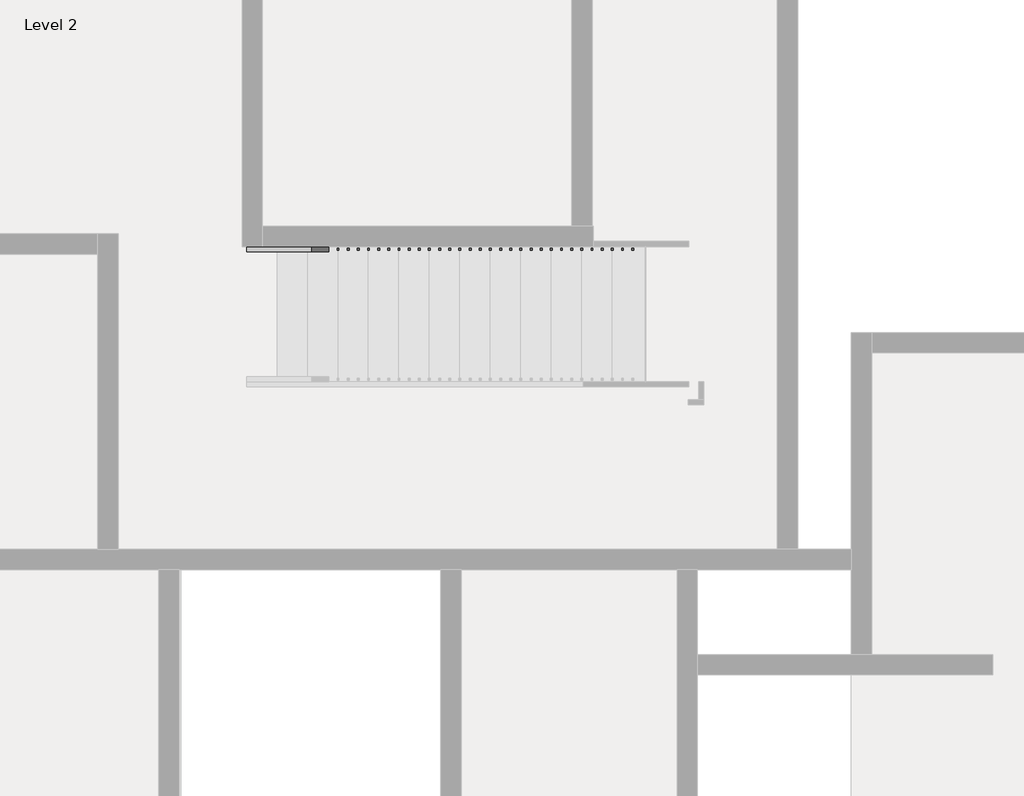
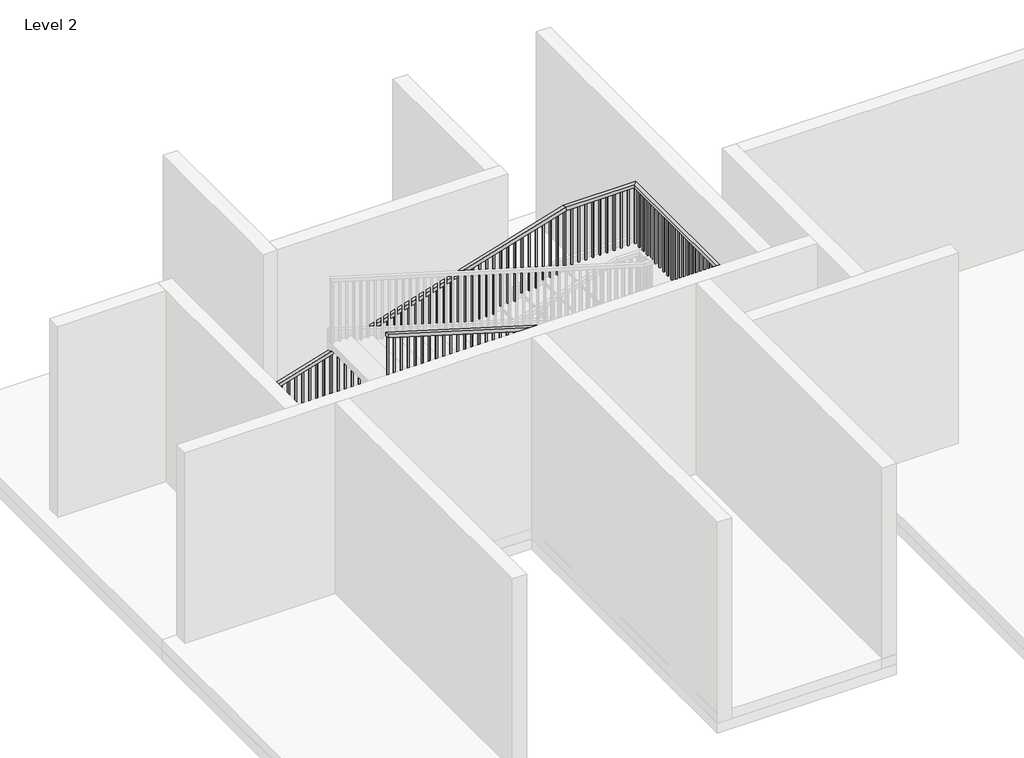
# One storey, part 10 of 14: 1 railing.
"""IFC4 building model written with IfcOpenShell, lengths in millimetres."""

from ifc_helpers import new_model, si_unit, frame, origin, place, context, project, spatial, polyline, outline, extrude, faceted_brep, element, save

model = new_model("IFC4")

# Units and contexts
model_context = context("Model", 3, world=origin())
ifc_project = project(units=[si_unit("LENGTHUNIT", "METRE", prefix="MILLI")], contexts=[model_context])

# Site, building, storey
site = spatial("IfcSite", under=ifc_project)
building = spatial("IfcBuilding", under=site)
storey = spatial("IfcBuildingStorey", under=building, Name="Level 2", Elevation=3048.0)

# Railing
placement = place(None, origin())
element("IfcRailing", 1, ObjectType="Handrail - Rectangular", at=placement, inside=storey, context=model_context, shape_type="SolidModel", body=[
    faceted_brep([(-5254.0891351, 12506.0715905, 4053.84), (-5254.0891351, 12506.0715905, 4000.8032429), (-5254.0891351, 12455.2715905, 4000.8032429), (-5254.0891351, 12455.2715905, 4053.84), (-986.8891351, 12506.0715905, 5334.0), (-979.4332782, 12506.0715905, 5283.2), (-979.4332782, 12455.2715905, 5283.2), (-986.8891351, 12455.2715905, 5334.0), (54.5108649, 12506.0715905, 5334.0), (54.5108649, 12506.0715905, 5283.2), (3.7108649, 12455.2715905, 5283.2), (3.7108649, 12455.2715905, 5334.0), (54.5108649, 9478.4949943, 5334.0), (54.5108649, 9478.4949943, 5283.2), (3.7108649, 9529.2949943, 5283.2), (3.7108649, 9529.2949943, 5334.0), (-682.0891351, 9478.4949943, 5334.0), (-689.544992, 9478.4949943, 5283.2), (-689.544992, 9529.2949943, 5283.2), (-682.0891351, 9529.2949943, 5334.0), (-5254.0891351, 9478.4949943, 6705.6), (-5254.0891351, 9529.2949943, 6705.6), (-5254.0891351, 9529.2949943, 6652.5632429), (-5254.0891351, 9478.4949943, 6652.5632429)], [[[0, 1, 2, 3]], [[1, 0, 4, 5]], [[2, 1, 5, 6]], [[3, 2, 6, 7]], [[0, 3, 7, 4]], [[5, 4, 8, 9]], [[6, 5, 9, 10]], [[7, 6, 10, 11]], [[4, 7, 11, 8]], [[9, 8, 12, 13]], [[10, 9, 13, 14]], [[11, 10, 14, 15]], [[8, 11, 15, 12]], [[13, 12, 16, 17]], [[14, 13, 17, 18]], [[15, 14, 18, 19]], [[12, 15, 19, 16]], [[20, 21, 22, 23]], [[17, 16, 20, 23]], [[18, 17, 23, 22]], [[19, 18, 22, 21]], [[16, 19, 21, 20]]]),
    extrude(outline(polyline([(6624.9407429, -5162.0141351), (5699.76, -5162.0141351), (5699.76, -5142.9641351), (6619.2257429, -5142.9641351), (6624.9407429, -5162.0141351)])), frame((0.0, 9494.3699943, 0.0), z_axis=(0.0, 1.0, 0.0), x_axis=(0.0, 0.0, 1.0)), (0.0, 0.0, 1.0), 19.05),
    extrude(outline(polyline([(6594.4607429, -5060.4141351), (5699.76, -5060.4141351), (5699.76, -5041.3641351), (6588.7457429, -5041.3641351), (6594.4607429, -5060.4141351)])), frame((0.0, 9494.3699943, 0.0), z_axis=(0.0, 1.0, 0.0), x_axis=(0.0, 0.0, 1.0)), (0.0, 0.0, 1.0), 19.05),
    extrude(outline(polyline([(6563.9807429, -4958.8141351), (5699.76, -4958.8141351), (5699.76, -4939.7641351), (6558.2657429, -4939.7641351), (6563.9807429, -4958.8141351)])), frame((0.0, 9494.3699943, 0.0), z_axis=(0.0, 1.0, 0.0), x_axis=(0.0, 0.0, 1.0)), (0.0, 0.0, 1.0), 19.05),
    extrude(outline(polyline([(6533.5007429, -4857.2141351), (5608.32, -4857.2141351), (5608.32, -4838.1641351), (6527.7857429, -4838.1641351), (6533.5007429, -4857.2141351)])), frame((0.0, 9494.3699943, 0.0), z_axis=(0.0, 1.0, 0.0), x_axis=(0.0, 0.0, 1.0)), (0.0, 0.0, 1.0), 19.05),
    extrude(outline(polyline([(6503.0207429, -4755.6141351), (5608.32, -4755.6141351), (5608.32, -4736.5641351), (6497.3057429, -4736.5641351), (6503.0207429, -4755.6141351)])), frame((0.0, 9494.3699943, 0.0), z_axis=(0.0, 1.0, 0.0), x_axis=(0.0, 0.0, 1.0)), (0.0, 0.0, 1.0), 19.05),
    extrude(outline(polyline([(6472.5407429, -4654.0141351), (5608.32, -4654.0141351), (5608.32, -4634.9641351), (6466.8257429, -4634.9641351), (6472.5407429, -4654.0141351)])), frame((0.0, 9494.3699943, 0.0), z_axis=(0.0, 1.0, 0.0), x_axis=(0.0, 0.0, 1.0)), (0.0, 0.0, 1.0), 19.05),
    extrude(outline(polyline([(6442.0607429, -4552.4141351), (5516.88, -4552.4141351), (5516.88, -4533.3641351), (6436.3457429, -4533.3641351), (6442.0607429, -4552.4141351)])), frame((0.0, 9494.3699943, 0.0), z_axis=(0.0, 1.0, 0.0), x_axis=(0.0, 0.0, 1.0)), (0.0, 0.0, 1.0), 19.05),
    extrude(outline(polyline([(6411.5807429, -4450.8141351), (5516.88, -4450.8141351), (5516.88, -4431.7641351), (6405.8657429, -4431.7641351), (6411.5807429, -4450.8141351)])), frame((0.0, 9494.3699943, 0.0), z_axis=(0.0, 1.0, 0.0), x_axis=(0.0, 0.0, 1.0)), (0.0, 0.0, 1.0), 19.05),
    extrude(outline(polyline([(6381.1007429, -4349.2141351), (5516.88, -4349.2141351), (5516.88, -4330.1641351), (6375.3857429, -4330.1641351), (6381.1007429, -4349.2141351)])), frame((0.0, 9494.3699943, 0.0), z_axis=(0.0, 1.0, 0.0), x_axis=(0.0, 0.0, 1.0)), (0.0, 0.0, 1.0), 19.05),
    extrude(outline(polyline([(6350.6207429, -4247.6141351), (5425.44, -4247.6141351), (5425.44, -4228.5641351), (6344.9057429, -4228.5641351), (6350.6207429, -4247.6141351)])), frame((0.0, 9494.3699943, 0.0), z_axis=(0.0, 1.0, 0.0), x_axis=(0.0, 0.0, 1.0)), (0.0, 0.0, 1.0), 19.05),
    extrude(outline(polyline([(6320.1407429, -4146.0141351), (5425.44, -4146.0141351), (5425.44, -4126.9641351), (6314.4257429, -4126.9641351), (6320.1407429, -4146.0141351)])), frame((0.0, 9494.3699943, 0.0), z_axis=(0.0, 1.0, 0.0), x_axis=(0.0, 0.0, 1.0)), (0.0, 0.0, 1.0), 19.05),
    extrude(outline(polyline([(6289.6607429, -4044.4141351), (5425.44, -4044.4141351), (5425.44, -4025.3641351), (6283.9457429, -4025.3641351), (6289.6607429, -4044.4141351)])), frame((0.0, 9494.3699943, 0.0), z_axis=(0.0, 1.0, 0.0), x_axis=(0.0, 0.0, 1.0)), (0.0, 0.0, 1.0), 19.05),
    extrude(outline(polyline([(6259.1807429, -3942.8141351), (5334.0, -3942.8141351), (5334.0, -3923.7641351), (6253.4657429, -3923.7641351), (6259.1807429, -3942.8141351)])), frame((0.0, 9494.3699943, 0.0), z_axis=(0.0, 1.0, 0.0), x_axis=(0.0, 0.0, 1.0)), (0.0, 0.0, 1.0), 19.05),
    extrude(outline(polyline([(6228.7007429, -3841.2141351), (5334.0, -3841.2141351), (5334.0, -3822.1641351), (6222.9857429, -3822.1641351), (6228.7007429, -3841.2141351)])), frame((0.0, 9494.3699943, 0.0), z_axis=(0.0, 1.0, 0.0), x_axis=(0.0, 0.0, 1.0)), (0.0, 0.0, 1.0), 19.05),
    extrude(outline(polyline([(6198.2207429, -3739.6141351), (5334.0, -3739.6141351), (5334.0, -3720.5641351), (6192.5057429, -3720.5641351), (6198.2207429, -3739.6141351)])), frame((0.0, 9494.3699943, 0.0), z_axis=(0.0, 1.0, 0.0), x_axis=(0.0, 0.0, 1.0)), (0.0, 0.0, 1.0), 19.05),
    extrude(outline(polyline([(6167.7407429, -3638.0141351), (5242.56, -3638.0141351), (5242.56, -3618.9641351), (6162.0257429, -3618.9641351), (6167.7407429, -3638.0141351)])), frame((0.0, 9494.3699943, 0.0), z_axis=(0.0, 1.0, 0.0), x_axis=(0.0, 0.0, 1.0)), (0.0, 0.0, 1.0), 19.05),
    extrude(outline(polyline([(6137.2607429, -3536.4141351), (5242.56, -3536.4141351), (5242.56, -3517.3641351), (6131.5457429, -3517.3641351), (6137.2607429, -3536.4141351)])), frame((0.0, 9494.3699943, 0.0), z_axis=(0.0, 1.0, 0.0), x_axis=(0.0, 0.0, 1.0)), (0.0, 0.0, 1.0), 19.05),
    extrude(outline(polyline([(6106.7807429, -3434.8141351), (5242.56, -3434.8141351), (5242.56, -3415.7641351), (6101.0657429, -3415.7641351), (6106.7807429, -3434.8141351)])), frame((0.0, 9494.3699943, 0.0), z_axis=(0.0, 1.0, 0.0), x_axis=(0.0, 0.0, 1.0)), (0.0, 0.0, 1.0), 19.05),
    extrude(outline(polyline([(6076.3007429, -3333.2141351), (5151.12, -3333.2141351), (5151.12, -3314.1641351), (6070.5857429, -3314.1641351), (6076.3007429, -3333.2141351)])), frame((0.0, 9494.3699943, 0.0), z_axis=(0.0, 1.0, 0.0), x_axis=(0.0, 0.0, 1.0)), (0.0, 0.0, 1.0), 19.05),
    extrude(outline(polyline([(6045.8207429, -3231.6141351), (5151.12, -3231.6141351), (5151.12, -3212.5641351), (6040.1057429, -3212.5641351), (6045.8207429, -3231.6141351)])), frame((0.0, 9494.3699943, 0.0), z_axis=(0.0, 1.0, 0.0), x_axis=(0.0, 0.0, 1.0)), (0.0, 0.0, 1.0), 19.05),
    extrude(outline(polyline([(6015.3407429, -3130.0141351), (5151.12, -3130.0141351), (5151.12, -3110.9641351), (6009.6257429, -3110.9641351), (6015.3407429, -3130.0141351)])), frame((0.0, 9494.3699943, 0.0), z_axis=(0.0, 1.0, 0.0), x_axis=(0.0, 0.0, 1.0)), (0.0, 0.0, 1.0), 19.05),
    extrude(outline(polyline([(5984.8607429, -3028.4141351), (5059.68, -3028.4141351), (5059.68, -3009.3641351), (5979.1457429, -3009.3641351), (5984.8607429, -3028.4141351)])), frame((0.0, 9494.3699943, 0.0), z_axis=(0.0, 1.0, 0.0), x_axis=(0.0, 0.0, 1.0)), (0.0, 0.0, 1.0), 19.05),
    extrude(outline(polyline([(5954.3807429, -2926.8141351), (5059.68, -2926.8141351), (5059.68, -2907.7641351), (5948.6657429, -2907.7641351), (5954.3807429, -2926.8141351)])), frame((0.0, 9494.3699943, 0.0), z_axis=(0.0, 1.0, 0.0), x_axis=(0.0, 0.0, 1.0)), (0.0, 0.0, 1.0), 19.05),
    extrude(outline(polyline([(5923.9007429, -2825.2141351), (5059.68, -2825.2141351), (5059.68, -2806.1641351), (5918.1857429, -2806.1641351), (5923.9007429, -2825.2141351)])), frame((0.0, 9494.3699943, 0.0), z_axis=(0.0, 1.0, 0.0), x_axis=(0.0, 0.0, 1.0)), (0.0, 0.0, 1.0), 19.05),
    extrude(outline(polyline([(5893.4207429, -2723.6141351), (4968.24, -2723.6141351), (4968.24, -2704.5641351), (5887.7057429, -2704.5641351), (5893.4207429, -2723.6141351)])), frame((0.0, 9494.3699943, 0.0), z_axis=(0.0, 1.0, 0.0), x_axis=(0.0, 0.0, 1.0)), (0.0, 0.0, 1.0), 19.05),
    extrude(outline(polyline([(5862.9407429, -2622.0141351), (4968.24, -2622.0141351), (4968.24, -2602.9641351), (5857.2257429, -2602.9641351), (5862.9407429, -2622.0141351)])), frame((0.0, 9494.3699943, 0.0), z_axis=(0.0, 1.0, 0.0), x_axis=(0.0, 0.0, 1.0)), (0.0, 0.0, 1.0), 19.05),
    extrude(outline(polyline([(5832.4607429, -2520.4141351), (4968.24, -2520.4141351), (4968.24, -2501.3641351), (5826.7457429, -2501.3641351), (5832.4607429, -2520.4141351)])), frame((0.0, 9494.3699943, 0.0), z_axis=(0.0, 1.0, 0.0), x_axis=(0.0, 0.0, 1.0)), (0.0, 0.0, 1.0), 19.05),
    extrude(outline(polyline([(5801.9807429, -2418.8141351), (4876.8, -2418.8141351), (4876.8, -2399.7641351), (5796.2657429, -2399.7641351), (5801.9807429, -2418.8141351)])), frame((0.0, 9494.3699943, 0.0), z_axis=(0.0, 1.0, 0.0), x_axis=(0.0, 0.0, 1.0)), (0.0, 0.0, 1.0), 19.05),
    extrude(outline(polyline([(5771.5007429, -2317.2141351), (4876.8, -2317.2141351), (4876.8, -2298.1641351), (5765.7857429, -2298.1641351), (5771.5007429, -2317.2141351)])), frame((0.0, 9494.3699943, 0.0), z_axis=(0.0, 1.0, 0.0), x_axis=(0.0, 0.0, 1.0)), (0.0, 0.0, 1.0), 19.05),
    extrude(outline(polyline([(5741.0207429, -2215.6141351), (4876.8, -2215.6141351), (4876.8, -2196.5641351), (5735.3057429, -2196.5641351), (5741.0207429, -2215.6141351)])), frame((0.0, 9494.3699943, 0.0), z_axis=(0.0, 1.0, 0.0), x_axis=(0.0, 0.0, 1.0)), (0.0, 0.0, 1.0), 19.05),
    extrude(outline(polyline([(5710.5407429, -2114.0141351), (4785.36, -2114.0141351), (4785.36, -2094.9641351), (5704.8257429, -2094.9641351), (5710.5407429, -2114.0141351)])), frame((0.0, 9494.3699943, 0.0), z_axis=(0.0, 1.0, 0.0), x_axis=(0.0, 0.0, 1.0)), (0.0, 0.0, 1.0), 19.05),
    extrude(outline(polyline([(5680.0607429, -2012.4141351), (4785.36, -2012.4141351), (4785.36, -1993.3641351), (5674.3457429, -1993.3641351), (5680.0607429, -2012.4141351)])), frame((0.0, 9494.3699943, 0.0), z_axis=(0.0, 1.0, 0.0), x_axis=(0.0, 0.0, 1.0)), (0.0, 0.0, 1.0), 19.05),
    extrude(outline(polyline([(5649.5807429, -1910.8141351), (4785.36, -1910.8141351), (4785.36, -1891.7641351), (5643.8657429, -1891.7641351), (5649.5807429, -1910.8141351)])), frame((0.0, 9494.3699943, 0.0), z_axis=(0.0, 1.0, 0.0), x_axis=(0.0, 0.0, 1.0)), (0.0, 0.0, 1.0), 19.05),
    extrude(outline(polyline([(5619.1007429, -1809.2141351), (4693.92, -1809.2141351), (4693.92, -1790.1641351), (5613.3857429, -1790.1641351), (5619.1007429, -1809.2141351)])), frame((0.0, 9494.3699943, 0.0), z_axis=(0.0, 1.0, 0.0), x_axis=(0.0, 0.0, 1.0)), (0.0, 0.0, 1.0), 19.05),
    extrude(outline(polyline([(5588.6207429, -1707.6141351), (4693.92, -1707.6141351), (4693.92, -1688.5641351), (5582.9057429, -1688.5641351), (5588.6207429, -1707.6141351)])), frame((0.0, 9494.3699943, 0.0), z_axis=(0.0, 1.0, 0.0), x_axis=(0.0, 0.0, 1.0)), (0.0, 0.0, 1.0), 19.05),
    extrude(outline(polyline([(5558.1407429, -1606.0141351), (4693.92, -1606.0141351), (4693.92, -1586.9641351), (5552.4257429, -1586.9641351), (5558.1407429, -1606.0141351)])), frame((0.0, 9494.3699943, 0.0), z_axis=(0.0, 1.0, 0.0), x_axis=(0.0, 0.0, 1.0)), (0.0, 0.0, 1.0), 19.05),
    extrude(outline(polyline([(5527.6607429, -1504.4141351), (4602.48, -1504.4141351), (4602.48, -1485.3641351), (5521.9457429, -1485.3641351), (5527.6607429, -1504.4141351)])), frame((0.0, 9494.3699943, 0.0), z_axis=(0.0, 1.0, 0.0), x_axis=(0.0, 0.0, 1.0)), (0.0, 0.0, 1.0), 19.05),
    extrude(outline(polyline([(5497.1807429, -1402.8141351), (4602.48, -1402.8141351), (4602.48, -1383.7641351), (5491.4657429, -1383.7641351), (5497.1807429, -1402.8141351)])), frame((0.0, 9494.3699943, 0.0), z_axis=(0.0, 1.0, 0.0), x_axis=(0.0, 0.0, 1.0)), (0.0, 0.0, 1.0), 19.05),
    extrude(outline(polyline([(5466.7007429, -1301.2141351), (4602.48, -1301.2141351), (4602.48, -1282.1641351), (5460.9857429, -1282.1641351), (5466.7007429, -1301.2141351)])), frame((0.0, 9494.3699943, 0.0), z_axis=(0.0, 1.0, 0.0), x_axis=(0.0, 0.0, 1.0)), (0.0, 0.0, 1.0), 19.05),
    extrude(outline(polyline([(5436.2207429, -1199.6141351), (4511.04, -1199.6141351), (4511.04, -1180.5641351), (5430.5057429, -1180.5641351), (5436.2207429, -1199.6141351)])), frame((0.0, 9494.3699943, 0.0), z_axis=(0.0, 1.0, 0.0), x_axis=(0.0, 0.0, 1.0)), (0.0, 0.0, 1.0), 19.05),
    extrude(outline(polyline([(5405.7407429, -1098.0141351), (4511.04, -1098.0141351), (4511.04, -1078.9641351), (5400.0257429, -1078.9641351), (5405.7407429, -1098.0141351)])), frame((0.0, 9494.3699943, 0.0), z_axis=(0.0, 1.0, 0.0), x_axis=(0.0, 0.0, 1.0)), (0.0, 0.0, 1.0), 19.05),
    extrude(outline(polyline([(5375.2607429, -996.4141351), (4511.04, -996.4141351), (4511.04, -977.3641351), (5369.5457429, -977.3641351), (5375.2607429, -996.4141351)])), frame((0.0, 9494.3699943, 0.0), z_axis=(0.0, 1.0, 0.0), x_axis=(0.0, 0.0, 1.0)), (0.0, 0.0, 1.0), 19.05),
    extrude(outline(polyline([(5344.7807429, -894.8141351), (4419.6, -894.8141351), (4419.6, -875.7641351), (5339.0657429, -875.7641351), (5344.7807429, -894.8141351)])), frame((0.0, 9494.3699943, 0.0), z_axis=(0.0, 1.0, 0.0), x_axis=(0.0, 0.0, 1.0)), (0.0, 0.0, 1.0), 19.05),
    extrude(outline(polyline([(5314.3007429, -793.2141351), (4419.6, -793.2141351), (4419.6, -774.1641351), (5308.5857429, -774.1641351), (5314.3007429, -793.2141351)])), frame((0.0, 9494.3699943, 0.0), z_axis=(0.0, 1.0, 0.0), x_axis=(0.0, 0.0, 1.0)), (0.0, 0.0, 1.0), 19.05),
    extrude(outline(polyline([(-672.5641351, 9494.3699943), (-691.6141351, 9494.3699943), (-691.6141351, 9513.4199943), (-672.5641351, 9513.4199943), (-672.5641351, 9494.3699943)])), frame((0.0, 0.0, 4419.6), z_axis=(0.0, 0.0, 1.0), x_axis=(1.0, 0.0, 0.0)), (0.0, 0.0, 1.0), 863.6),
    extrude(outline(polyline([(-570.9641351, 9494.3699943), (-590.0141351, 9494.3699943), (-590.0141351, 9513.4199943), (-570.9641351, 9513.4199943), (-570.9641351, 9494.3699943)])), frame((0.0, 0.0, 4419.6), z_axis=(0.0, 0.0, 1.0), x_axis=(1.0, 0.0, 0.0)), (0.0, 0.0, 1.0), 863.6),
    extrude(outline(polyline([(-469.3641351, 9494.3699943), (-488.4141351, 9494.3699943), (-488.4141351, 9513.4199943), (-469.3641351, 9513.4199943), (-469.3641351, 9494.3699943)])), frame((0.0, 0.0, 4419.6), z_axis=(0.0, 0.0, 1.0), x_axis=(1.0, 0.0, 0.0)), (0.0, 0.0, 1.0), 863.6),
    extrude(outline(polyline([(-367.7641351, 9494.3699943), (-386.8141351, 9494.3699943), (-386.8141351, 9513.4199943), (-367.7641351, 9513.4199943), (-367.7641351, 9494.3699943)])), frame((0.0, 0.0, 4419.6), z_axis=(0.0, 0.0, 1.0), x_axis=(1.0, 0.0, 0.0)), (0.0, 0.0, 1.0), 863.6),
    extrude(outline(polyline([(-266.1641351, 9494.3699943), (-285.2141351, 9494.3699943), (-285.2141351, 9513.4199943), (-266.1641351, 9513.4199943), (-266.1641351, 9494.3699943)])), frame((0.0, 0.0, 4419.6), z_axis=(0.0, 0.0, 1.0), x_axis=(1.0, 0.0, 0.0)), (0.0, 0.0, 1.0), 863.6),
    extrude(outline(polyline([(-164.5641351, 9494.3699943), (-183.6141351, 9494.3699943), (-183.6141351, 9513.4199943), (-164.5641351, 9513.4199943), (-164.5641351, 9494.3699943)])), frame((0.0, 0.0, 4419.6), z_axis=(0.0, 0.0, 1.0), x_axis=(1.0, 0.0, 0.0)), (0.0, 0.0, 1.0), 863.6),
    extrude(outline(polyline([(-62.9641351, 9494.3699943), (-82.0141351, 9494.3699943), (-82.0141351, 9513.4199943), (-62.9641351, 9513.4199943), (-62.9641351, 9494.3699943)])), frame((0.0, 0.0, 4419.6), z_axis=(0.0, 0.0, 1.0), x_axis=(1.0, 0.0, 0.0)), (0.0, 0.0, 1.0), 863.6),
    extrude(outline(polyline([(38.6358649, 9543.7965905), (38.6358649, 9524.7465905), (19.5858649, 9524.7465905), (19.5858649, 9543.7965905), (38.6358649, 9543.7965905)])), frame((0.0, 0.0, 4419.6), z_axis=(0.0, 0.0, 1.0), x_axis=(1.0, 0.0, 0.0)), (0.0, 0.0, 1.0), 863.6),
    extrude(outline(polyline([(38.6358649, 9645.3965905), (38.6358649, 9626.3465905), (19.5858649, 9626.3465905), (19.5858649, 9645.3965905), (38.6358649, 9645.3965905)])), frame((0.0, 0.0, 4419.6), z_axis=(0.0, 0.0, 1.0), x_axis=(1.0, 0.0, 0.0)), (0.0, 0.0, 1.0), 863.6),
    extrude(outline(polyline([(38.6358649, 9746.9965905), (38.6358649, 9727.9465905), (19.5858649, 9727.9465905), (19.5858649, 9746.9965905), (38.6358649, 9746.9965905)])), frame((0.0, 0.0, 4419.6), z_axis=(0.0, 0.0, 1.0), x_axis=(1.0, 0.0, 0.0)), (0.0, 0.0, 1.0), 863.6),
    extrude(outline(polyline([(38.6358649, 9848.5965905), (38.6358649, 9829.5465905), (19.5858649, 9829.5465905), (19.5858649, 9848.5965905), (38.6358649, 9848.5965905)])), frame((0.0, 0.0, 4419.6), z_axis=(0.0, 0.0, 1.0), x_axis=(1.0, 0.0, 0.0)), (0.0, 0.0, 1.0), 863.6),
    extrude(outline(polyline([(38.6358649, 9950.1965905), (38.6358649, 9931.1465905), (19.5858649, 9931.1465905), (19.5858649, 9950.1965905), (38.6358649, 9950.1965905)])), frame((0.0, 0.0, 4419.6), z_axis=(0.0, 0.0, 1.0), x_axis=(1.0, 0.0, 0.0)), (0.0, 0.0, 1.0), 863.6),
    extrude(outline(polyline([(38.6358649, 10051.7965905), (38.6358649, 10032.7465905), (19.5858649, 10032.7465905), (19.5858649, 10051.7965905), (38.6358649, 10051.7965905)])), frame((0.0, 0.0, 4419.6), z_axis=(0.0, 0.0, 1.0), x_axis=(1.0, 0.0, 0.0)), (0.0, 0.0, 1.0), 863.6),
    extrude(outline(polyline([(38.6358649, 10153.3965905), (38.6358649, 10134.3465905), (19.5858649, 10134.3465905), (19.5858649, 10153.3965905), (38.6358649, 10153.3965905)])), frame((0.0, 0.0, 4419.6), z_axis=(0.0, 0.0, 1.0), x_axis=(1.0, 0.0, 0.0)), (0.0, 0.0, 1.0), 863.6),
    extrude(outline(polyline([(38.6358649, 10254.9965905), (38.6358649, 10235.9465905), (19.5858649, 10235.9465905), (19.5858649, 10254.9965905), (38.6358649, 10254.9965905)])), frame((0.0, 0.0, 4419.6), z_axis=(0.0, 0.0, 1.0), x_axis=(1.0, 0.0, 0.0)), (0.0, 0.0, 1.0), 863.6),
    extrude(outline(polyline([(38.6358649, 10356.5965905), (38.6358649, 10337.5465905), (19.5858649, 10337.5465905), (19.5858649, 10356.5965905), (38.6358649, 10356.5965905)])), frame((0.0, 0.0, 4419.6), z_axis=(0.0, 0.0, 1.0), x_axis=(1.0, 0.0, 0.0)), (0.0, 0.0, 1.0), 863.6),
    extrude(outline(polyline([(38.6358649, 10458.1965905), (38.6358649, 10439.1465905), (19.5858649, 10439.1465905), (19.5858649, 10458.1965905), (38.6358649, 10458.1965905)])), frame((0.0, 0.0, 4419.6), z_axis=(0.0, 0.0, 1.0), x_axis=(1.0, 0.0, 0.0)), (0.0, 0.0, 1.0), 863.6),
    extrude(outline(polyline([(38.6358649, 10559.7965905), (38.6358649, 10540.7465905), (19.5858649, 10540.7465905), (19.5858649, 10559.7965905), (38.6358649, 10559.7965905)])), frame((0.0, 0.0, 4419.6), z_axis=(0.0, 0.0, 1.0), x_axis=(1.0, 0.0, 0.0)), (0.0, 0.0, 1.0), 863.6),
    extrude(outline(polyline([(38.6358649, 10661.3965905), (38.6358649, 10642.3465905), (19.5858649, 10642.3465905), (19.5858649, 10661.3965905), (38.6358649, 10661.3965905)])), frame((0.0, 0.0, 4419.6), z_axis=(0.0, 0.0, 1.0), x_axis=(1.0, 0.0, 0.0)), (0.0, 0.0, 1.0), 863.6),
    extrude(outline(polyline([(38.6358649, 10762.9965905), (38.6358649, 10743.9465905), (19.5858649, 10743.9465905), (19.5858649, 10762.9965905), (38.6358649, 10762.9965905)])), frame((0.0, 0.0, 4419.6), z_axis=(0.0, 0.0, 1.0), x_axis=(1.0, 0.0, 0.0)), (0.0, 0.0, 1.0), 863.6),
    extrude(outline(polyline([(38.6358649, 10864.5965905), (38.6358649, 10845.5465905), (19.5858649, 10845.5465905), (19.5858649, 10864.5965905), (38.6358649, 10864.5965905)])), frame((0.0, 0.0, 4419.6), z_axis=(0.0, 0.0, 1.0), x_axis=(1.0, 0.0, 0.0)), (0.0, 0.0, 1.0), 863.6),
    extrude(outline(polyline([(38.6358649, 10966.1965905), (38.6358649, 10947.1465905), (19.5858649, 10947.1465905), (19.5858649, 10966.1965905), (38.6358649, 10966.1965905)])), frame((0.0, 0.0, 4419.6), z_axis=(0.0, 0.0, 1.0), x_axis=(1.0, 0.0, 0.0)), (0.0, 0.0, 1.0), 863.6),
    extrude(outline(polyline([(38.6358649, 11067.7965905), (38.6358649, 11048.7465905), (19.5858649, 11048.7465905), (19.5858649, 11067.7965905), (38.6358649, 11067.7965905)])), frame((0.0, 0.0, 4419.6), z_axis=(0.0, 0.0, 1.0), x_axis=(1.0, 0.0, 0.0)), (0.0, 0.0, 1.0), 863.6),
    extrude(outline(polyline([(38.6358649, 11169.3965905), (38.6358649, 11150.3465905), (19.5858649, 11150.3465905), (19.5858649, 11169.3965905), (38.6358649, 11169.3965905)])), frame((0.0, 0.0, 4419.6), z_axis=(0.0, 0.0, 1.0), x_axis=(1.0, 0.0, 0.0)), (0.0, 0.0, 1.0), 863.6),
    extrude(outline(polyline([(38.6358649, 11270.9965905), (38.6358649, 11251.9465905), (19.5858649, 11251.9465905), (19.5858649, 11270.9965905), (38.6358649, 11270.9965905)])), frame((0.0, 0.0, 4419.6), z_axis=(0.0, 0.0, 1.0), x_axis=(1.0, 0.0, 0.0)), (0.0, 0.0, 1.0), 863.6),
    extrude(outline(polyline([(38.6358649, 11372.5965905), (38.6358649, 11353.5465905), (19.5858649, 11353.5465905), (19.5858649, 11372.5965905), (38.6358649, 11372.5965905)])), frame((0.0, 0.0, 4419.6), z_axis=(0.0, 0.0, 1.0), x_axis=(1.0, 0.0, 0.0)), (0.0, 0.0, 1.0), 863.6),
    extrude(outline(polyline([(38.6358649, 11474.1965905), (38.6358649, 11455.1465905), (19.5858649, 11455.1465905), (19.5858649, 11474.1965905), (38.6358649, 11474.1965905)])), frame((0.0, 0.0, 4419.6), z_axis=(0.0, 0.0, 1.0), x_axis=(1.0, 0.0, 0.0)), (0.0, 0.0, 1.0), 863.6),
    extrude(outline(polyline([(38.6358649, 11575.7965905), (38.6358649, 11556.7465905), (19.5858649, 11556.7465905), (19.5858649, 11575.7965905), (38.6358649, 11575.7965905)])), frame((0.0, 0.0, 4419.6), z_axis=(0.0, 0.0, 1.0), x_axis=(1.0, 0.0, 0.0)), (0.0, 0.0, 1.0), 863.6),
    extrude(outline(polyline([(38.6358649, 11677.3965905), (38.6358649, 11658.3465905), (19.5858649, 11658.3465905), (19.5858649, 11677.3965905), (38.6358649, 11677.3965905)])), frame((0.0, 0.0, 4419.6), z_axis=(0.0, 0.0, 1.0), x_axis=(1.0, 0.0, 0.0)), (0.0, 0.0, 1.0), 863.6),
    extrude(outline(polyline([(38.6358649, 11778.9965905), (38.6358649, 11759.9465905), (19.5858649, 11759.9465905), (19.5858649, 11778.9965905), (38.6358649, 11778.9965905)])), frame((0.0, 0.0, 4419.6), z_axis=(0.0, 0.0, 1.0), x_axis=(1.0, 0.0, 0.0)), (0.0, 0.0, 1.0), 863.6),
    extrude(outline(polyline([(38.6358649, 11880.5965905), (38.6358649, 11861.5465905), (19.5858649, 11861.5465905), (19.5858649, 11880.5965905), (38.6358649, 11880.5965905)])), frame((0.0, 0.0, 4419.6), z_axis=(0.0, 0.0, 1.0), x_axis=(1.0, 0.0, 0.0)), (0.0, 0.0, 1.0), 863.6),
    extrude(outline(polyline([(38.6358649, 11982.1965905), (38.6358649, 11963.1465905), (19.5858649, 11963.1465905), (19.5858649, 11982.1965905), (38.6358649, 11982.1965905)])), frame((0.0, 0.0, 4419.6), z_axis=(0.0, 0.0, 1.0), x_axis=(1.0, 0.0, 0.0)), (0.0, 0.0, 1.0), 863.6),
    extrude(outline(polyline([(38.6358649, 12083.7965905), (38.6358649, 12064.7465905), (19.5858649, 12064.7465905), (19.5858649, 12083.7965905), (38.6358649, 12083.7965905)])), frame((0.0, 0.0, 4419.6), z_axis=(0.0, 0.0, 1.0), x_axis=(1.0, 0.0, 0.0)), (0.0, 0.0, 1.0), 863.6),
    extrude(outline(polyline([(38.6358649, 12185.3965905), (38.6358649, 12166.3465905), (19.5858649, 12166.3465905), (19.5858649, 12185.3965905), (38.6358649, 12185.3965905)])), frame((0.0, 0.0, 4419.6), z_axis=(0.0, 0.0, 1.0), x_axis=(1.0, 0.0, 0.0)), (0.0, 0.0, 1.0), 863.6),
    extrude(outline(polyline([(38.6358649, 12286.9965905), (38.6358649, 12267.9465905), (19.5858649, 12267.9465905), (19.5858649, 12286.9965905), (38.6358649, 12286.9965905)])), frame((0.0, 0.0, 4419.6), z_axis=(0.0, 0.0, 1.0), x_axis=(1.0, 0.0, 0.0)), (0.0, 0.0, 1.0), 863.6),
    extrude(outline(polyline([(38.6358649, 12388.5965905), (38.6358649, 12369.5465905), (19.5858649, 12369.5465905), (19.5858649, 12388.5965905), (38.6358649, 12388.5965905)])), frame((0.0, 0.0, 4419.6), z_axis=(0.0, 0.0, 1.0), x_axis=(1.0, 0.0, 0.0)), (0.0, 0.0, 1.0), 863.6),
    extrude(outline(polyline([(-82.0141351, 12490.1965905), (-62.9641351, 12490.1965905), (-62.9641351, 12471.1465905), (-82.0141351, 12471.1465905), (-82.0141351, 12490.1965905)])), frame((0.0, 0.0, 4419.6), z_axis=(0.0, 0.0, 1.0), x_axis=(1.0, 0.0, 0.0)), (0.0, 0.0, 1.0), 863.6),
    extrude(outline(polyline([(-183.6141351, 12490.1965905), (-164.5641351, 12490.1965905), (-164.5641351, 12471.1465905), (-183.6141351, 12471.1465905), (-183.6141351, 12490.1965905)])), frame((0.0, 0.0, 4419.6), z_axis=(0.0, 0.0, 1.0), x_axis=(1.0, 0.0, 0.0)), (0.0, 0.0, 1.0), 863.6),
    extrude(outline(polyline([(-285.2141351, 12490.1965905), (-266.1641351, 12490.1965905), (-266.1641351, 12471.1465905), (-285.2141351, 12471.1465905), (-285.2141351, 12490.1965905)])), frame((0.0, 0.0, 4419.6), z_axis=(0.0, 0.0, 1.0), x_axis=(1.0, 0.0, 0.0)), (0.0, 0.0, 1.0), 863.6),
    extrude(outline(polyline([(-386.8141351, 12490.1965905), (-367.7641351, 12490.1965905), (-367.7641351, 12471.1465905), (-386.8141351, 12471.1465905), (-386.8141351, 12490.1965905)])), frame((0.0, 0.0, 4419.6), z_axis=(0.0, 0.0, 1.0), x_axis=(1.0, 0.0, 0.0)), (0.0, 0.0, 1.0), 863.6),
    extrude(outline(polyline([(-488.4141351, 12490.1965905), (-469.3641351, 12490.1965905), (-469.3641351, 12471.1465905), (-488.4141351, 12471.1465905), (-488.4141351, 12490.1965905)])), frame((0.0, 0.0, 4419.6), z_axis=(0.0, 0.0, 1.0), x_axis=(1.0, 0.0, 0.0)), (0.0, 0.0, 1.0), 863.6),
    extrude(outline(polyline([(-590.0141351, 12490.1965905), (-570.9641351, 12490.1965905), (-570.9641351, 12471.1465905), (-590.0141351, 12471.1465905), (-590.0141351, 12490.1965905)])), frame((0.0, 0.0, 4419.6), z_axis=(0.0, 0.0, 1.0), x_axis=(1.0, 0.0, 0.0)), (0.0, 0.0, 1.0), 863.6),
    extrude(outline(polyline([(-691.6141351, 12490.1965905), (-672.5641351, 12490.1965905), (-672.5641351, 12471.1465905), (-691.6141351, 12471.1465905), (-691.6141351, 12490.1965905)])), frame((0.0, 0.0, 4419.6), z_axis=(0.0, 0.0, 1.0), x_axis=(1.0, 0.0, 0.0)), (0.0, 0.0, 1.0), 863.6),
    extrude(outline(polyline([(-793.2141351, 12490.1965905), (-774.1641351, 12490.1965905), (-774.1641351, 12471.1465905), (-793.2141351, 12471.1465905), (-793.2141351, 12490.1965905)])), frame((0.0, 0.0, 4419.6), z_axis=(0.0, 0.0, 1.0), x_axis=(1.0, 0.0, 0.0)), (0.0, 0.0, 1.0), 863.6),
    extrude(outline(polyline([(-894.8141351, 12490.1965905), (-875.7641351, 12490.1965905), (-875.7641351, 12471.1465905), (-894.8141351, 12471.1465905), (-894.8141351, 12490.1965905)])), frame((0.0, 0.0, 4419.6), z_axis=(0.0, 0.0, 1.0), x_axis=(1.0, 0.0, 0.0)), (0.0, 0.0, 1.0), 863.6),
    extrude(outline(polyline([(5278.1057429, -996.4141351), (4419.6, -996.4141351), (4419.6, -977.3641351), (5283.8207429, -977.3641351), (5278.1057429, -996.4141351)])), frame((0.0, 12471.1465905, 0.0), z_axis=(0.0, 1.0, 0.0), x_axis=(0.0, 0.0, 1.0)), (0.0, 0.0, 1.0), 19.05),
    extrude(outline(polyline([(5247.6257429, -1098.0141351), (4328.16, -1098.0141351), (4328.16, -1078.9641351), (5253.3407429, -1078.9641351), (5247.6257429, -1098.0141351)])), frame((0.0, 12471.1465905, 0.0), z_axis=(0.0, 1.0, 0.0), x_axis=(0.0, 0.0, 1.0)), (0.0, 0.0, 1.0), 19.05),
    extrude(outline(polyline([(5217.1457429, -1199.6141351), (4328.16, -1199.6141351), (4328.16, -1180.5641351), (5222.8607429, -1180.5641351), (5217.1457429, -1199.6141351)])), frame((0.0, 12471.1465905, 0.0), z_axis=(0.0, 1.0, 0.0), x_axis=(0.0, 0.0, 1.0)), (0.0, 0.0, 1.0), 19.05),
    extrude(outline(polyline([(5186.6657429, -1301.2141351), (4328.16, -1301.2141351), (4328.16, -1282.1641351), (5192.3807429, -1282.1641351), (5186.6657429, -1301.2141351)])), frame((0.0, 12471.1465905, 0.0), z_axis=(0.0, 1.0, 0.0), x_axis=(0.0, 0.0, 1.0)), (0.0, 0.0, 1.0), 19.05),
    extrude(outline(polyline([(5156.1857429, -1402.8141351), (4236.72, -1402.8141351), (4236.72, -1383.7641351), (5161.9007429, -1383.7641351), (5156.1857429, -1402.8141351)])), frame((0.0, 12471.1465905, 0.0), z_axis=(0.0, 1.0, 0.0), x_axis=(0.0, 0.0, 1.0)), (0.0, 0.0, 1.0), 19.05),
    extrude(outline(polyline([(5125.7057429, -1504.4141351), (4236.72, -1504.4141351), (4236.72, -1485.3641351), (5131.4207429, -1485.3641351), (5125.7057429, -1504.4141351)])), frame((0.0, 12471.1465905, 0.0), z_axis=(0.0, 1.0, 0.0), x_axis=(0.0, 0.0, 1.0)), (0.0, 0.0, 1.0), 19.05),
    extrude(outline(polyline([(5095.2257429, -1606.0141351), (4236.72, -1606.0141351), (4236.72, -1586.9641351), (5100.9407429, -1586.9641351), (5095.2257429, -1606.0141351)])), frame((0.0, 12471.1465905, 0.0), z_axis=(0.0, 1.0, 0.0), x_axis=(0.0, 0.0, 1.0)), (0.0, 0.0, 1.0), 19.05),
    extrude(outline(polyline([(5064.7457429, -1707.6141351), (4145.28, -1707.6141351), (4145.28, -1688.5641351), (5070.4607429, -1688.5641351), (5064.7457429, -1707.6141351)])), frame((0.0, 12471.1465905, 0.0), z_axis=(0.0, 1.0, 0.0), x_axis=(0.0, 0.0, 1.0)), (0.0, 0.0, 1.0), 19.05),
    extrude(outline(polyline([(5034.2657429, -1809.2141351), (4145.28, -1809.2141351), (4145.28, -1790.1641351), (5039.9807429, -1790.1641351), (5034.2657429, -1809.2141351)])), frame((0.0, 12471.1465905, 0.0), z_axis=(0.0, 1.0, 0.0), x_axis=(0.0, 0.0, 1.0)), (0.0, 0.0, 1.0), 19.05),
    extrude(outline(polyline([(5003.7857429, -1910.8141351), (4145.28, -1910.8141351), (4145.28, -1891.7641351), (5009.5007429, -1891.7641351), (5003.7857429, -1910.8141351)])), frame((0.0, 12471.1465905, 0.0), z_axis=(0.0, 1.0, 0.0), x_axis=(0.0, 0.0, 1.0)), (0.0, 0.0, 1.0), 19.05),
    extrude(outline(polyline([(4973.3057429, -2012.4141351), (4053.84, -2012.4141351), (4053.84, -1993.3641351), (4979.0207429, -1993.3641351), (4973.3057429, -2012.4141351)])), frame((0.0, 12471.1465905, 0.0), z_axis=(0.0, 1.0, 0.0), x_axis=(0.0, 0.0, 1.0)), (0.0, 0.0, 1.0), 19.05),
    extrude(outline(polyline([(4942.8257429, -2114.0141351), (4053.84, -2114.0141351), (4053.84, -2094.9641351), (4948.5407429, -2094.9641351), (4942.8257429, -2114.0141351)])), frame((0.0, 12471.1465905, 0.0), z_axis=(0.0, 1.0, 0.0), x_axis=(0.0, 0.0, 1.0)), (0.0, 0.0, 1.0), 19.05),
    extrude(outline(polyline([(4912.3457429, -2215.6141351), (4053.84, -2215.6141351), (4053.84, -2196.5641351), (4918.0607429, -2196.5641351), (4912.3457429, -2215.6141351)])), frame((0.0, 12471.1465905, 0.0), z_axis=(0.0, 1.0, 0.0), x_axis=(0.0, 0.0, 1.0)), (0.0, 0.0, 1.0), 19.05),
    extrude(outline(polyline([(4881.8657429, -2317.2141351), (3962.4, -2317.2141351), (3962.4, -2298.1641351), (4887.5807429, -2298.1641351), (4881.8657429, -2317.2141351)])), frame((0.0, 12471.1465905, 0.0), z_axis=(0.0, 1.0, 0.0), x_axis=(0.0, 0.0, 1.0)), (0.0, 0.0, 1.0), 19.05),
    extrude(outline(polyline([(4851.3857429, -2418.8141351), (3962.4, -2418.8141351), (3962.4, -2399.7641351), (4857.1007429, -2399.7641351), (4851.3857429, -2418.8141351)])), frame((0.0, 12471.1465905, 0.0), z_axis=(0.0, 1.0, 0.0), x_axis=(0.0, 0.0, 1.0)), (0.0, 0.0, 1.0), 19.05),
    extrude(outline(polyline([(4820.9057429, -2520.4141351), (3962.4, -2520.4141351), (3962.4, -2501.3641351), (4826.6207429, -2501.3641351), (4820.9057429, -2520.4141351)])), frame((0.0, 12471.1465905, 0.0), z_axis=(0.0, 1.0, 0.0), x_axis=(0.0, 0.0, 1.0)), (0.0, 0.0, 1.0), 19.05),
    extrude(outline(polyline([(4790.4257429, -2622.0141351), (3870.96, -2622.0141351), (3870.96, -2602.9641351), (4796.1407429, -2602.9641351), (4790.4257429, -2622.0141351)])), frame((0.0, 12471.1465905, 0.0), z_axis=(0.0, 1.0, 0.0), x_axis=(0.0, 0.0, 1.0)), (0.0, 0.0, 1.0), 19.05),
    extrude(outline(polyline([(4759.9457429, -2723.6141351), (3870.96, -2723.6141351), (3870.96, -2704.5641351), (4765.6607429, -2704.5641351), (4759.9457429, -2723.6141351)])), frame((0.0, 12471.1465905, 0.0), z_axis=(0.0, 1.0, 0.0), x_axis=(0.0, 0.0, 1.0)), (0.0, 0.0, 1.0), 19.05),
    extrude(outline(polyline([(4729.4657429, -2825.2141351), (3870.96, -2825.2141351), (3870.96, -2806.1641351), (4735.1807429, -2806.1641351), (4729.4657429, -2825.2141351)])), frame((0.0, 12471.1465905, 0.0), z_axis=(0.0, 1.0, 0.0), x_axis=(0.0, 0.0, 1.0)), (0.0, 0.0, 1.0), 19.05),
    extrude(outline(polyline([(4698.9857429, -2926.8141351), (3779.52, -2926.8141351), (3779.52, -2907.7641351), (4704.7007429, -2907.7641351), (4698.9857429, -2926.8141351)])), frame((0.0, 12471.1465905, 0.0), z_axis=(0.0, 1.0, 0.0), x_axis=(0.0, 0.0, 1.0)), (0.0, 0.0, 1.0), 19.05),
    extrude(outline(polyline([(4668.5057429, -3028.4141351), (3779.52, -3028.4141351), (3779.52, -3009.3641351), (4674.2207429, -3009.3641351), (4668.5057429, -3028.4141351)])), frame((0.0, 12471.1465905, 0.0), z_axis=(0.0, 1.0, 0.0), x_axis=(0.0, 0.0, 1.0)), (0.0, 0.0, 1.0), 19.05),
    extrude(outline(polyline([(4638.0257429, -3130.0141351), (3779.52, -3130.0141351), (3779.52, -3110.9641351), (4643.7407429, -3110.9641351), (4638.0257429, -3130.0141351)])), frame((0.0, 12471.1465905, 0.0), z_axis=(0.0, 1.0, 0.0), x_axis=(0.0, 0.0, 1.0)), (0.0, 0.0, 1.0), 19.05),
    extrude(outline(polyline([(4607.5457429, -3231.6141351), (3688.08, -3231.6141351), (3688.08, -3212.5641351), (4613.2607429, -3212.5641351), (4607.5457429, -3231.6141351)])), frame((0.0, 12471.1465905, 0.0), z_axis=(0.0, 1.0, 0.0), x_axis=(0.0, 0.0, 1.0)), (0.0, 0.0, 1.0), 19.05),
    extrude(outline(polyline([(4577.0657429, -3333.2141351), (3688.08, -3333.2141351), (3688.08, -3314.1641351), (4582.7807429, -3314.1641351), (4577.0657429, -3333.2141351)])), frame((0.0, 12471.1465905, 0.0), z_axis=(0.0, 1.0, 0.0), x_axis=(0.0, 0.0, 1.0)), (0.0, 0.0, 1.0), 19.05),
    extrude(outline(polyline([(4546.5857429, -3434.8141351), (3688.08, -3434.8141351), (3688.08, -3415.7641351), (4552.3007429, -3415.7641351), (4546.5857429, -3434.8141351)])), frame((0.0, 12471.1465905, 0.0), z_axis=(0.0, 1.0, 0.0), x_axis=(0.0, 0.0, 1.0)), (0.0, 0.0, 1.0), 19.05),
    extrude(outline(polyline([(4516.1057429, -3536.4141351), (3596.64, -3536.4141351), (3596.64, -3517.3641351), (4521.8207429, -3517.3641351), (4516.1057429, -3536.4141351)])), frame((0.0, 12471.1465905, 0.0), z_axis=(0.0, 1.0, 0.0), x_axis=(0.0, 0.0, 1.0)), (0.0, 0.0, 1.0), 19.05),
    extrude(outline(polyline([(4485.6257429, -3638.0141351), (3596.64, -3638.0141351), (3596.64, -3618.9641351), (4491.3407429, -3618.9641351), (4485.6257429, -3638.0141351)])), frame((0.0, 12471.1465905, 0.0), z_axis=(0.0, 1.0, 0.0), x_axis=(0.0, 0.0, 1.0)), (0.0, 0.0, 1.0), 19.05),
    extrude(outline(polyline([(4455.1457429, -3739.6141351), (3596.64, -3739.6141351), (3596.64, -3720.5641351), (4460.8607429, -3720.5641351), (4455.1457429, -3739.6141351)])), frame((0.0, 12471.1465905, 0.0), z_axis=(0.0, 1.0, 0.0), x_axis=(0.0, 0.0, 1.0)), (0.0, 0.0, 1.0), 19.05),
    extrude(outline(polyline([(4424.6657429, -3841.2141351), (3505.2, -3841.2141351), (3505.2, -3822.1641351), (4430.3807429, -3822.1641351), (4424.6657429, -3841.2141351)])), frame((0.0, 12471.1465905, 0.0), z_axis=(0.0, 1.0, 0.0), x_axis=(0.0, 0.0, 1.0)), (0.0, 0.0, 1.0), 19.05),
    extrude(outline(polyline([(4394.1857429, -3942.8141351), (3505.2, -3942.8141351), (3505.2, -3923.7641351), (4399.9007429, -3923.7641351), (4394.1857429, -3942.8141351)])), frame((0.0, 12471.1465905, 0.0), z_axis=(0.0, 1.0, 0.0), x_axis=(0.0, 0.0, 1.0)), (0.0, 0.0, 1.0), 19.05),
    extrude(outline(polyline([(4363.7057429, -4044.4141351), (3505.2, -4044.4141351), (3505.2, -4025.3641351), (4369.4207429, -4025.3641351), (4363.7057429, -4044.4141351)])), frame((0.0, 12471.1465905, 0.0), z_axis=(0.0, 1.0, 0.0), x_axis=(0.0, 0.0, 1.0)), (0.0, 0.0, 1.0), 19.05),
    extrude(outline(polyline([(4333.2257429, -4146.0141351), (3413.76, -4146.0141351), (3413.76, -4126.9641351), (4338.9407429, -4126.9641351), (4333.2257429, -4146.0141351)])), frame((0.0, 12471.1465905, 0.0), z_axis=(0.0, 1.0, 0.0), x_axis=(0.0, 0.0, 1.0)), (0.0, 0.0, 1.0), 19.05),
    extrude(outline(polyline([(4302.7457429, -4247.6141351), (3413.76, -4247.6141351), (3413.76, -4228.5641351), (4308.4607429, -4228.5641351), (4302.7457429, -4247.6141351)])), frame((0.0, 12471.1465905, 0.0), z_axis=(0.0, 1.0, 0.0), x_axis=(0.0, 0.0, 1.0)), (0.0, 0.0, 1.0), 19.05),
    extrude(outline(polyline([(4272.2657429, -4349.2141351), (3413.76, -4349.2141351), (3413.76, -4330.1641351), (4277.9807429, -4330.1641351), (4272.2657429, -4349.2141351)])), frame((0.0, 12471.1465905, 0.0), z_axis=(0.0, 1.0, 0.0), x_axis=(0.0, 0.0, 1.0)), (0.0, 0.0, 1.0), 19.05),
    extrude(outline(polyline([(4241.7857429, -4450.8141351), (3322.32, -4450.8141351), (3322.32, -4431.7641351), (4247.5007429, -4431.7641351), (4241.7857429, -4450.8141351)])), frame((0.0, 12471.1465905, 0.0), z_axis=(0.0, 1.0, 0.0), x_axis=(0.0, 0.0, 1.0)), (0.0, 0.0, 1.0), 19.05),
    extrude(outline(polyline([(4211.3057429, -4552.4141351), (3322.32, -4552.4141351), (3322.32, -4533.3641351), (4217.0207429, -4533.3641351), (4211.3057429, -4552.4141351)])), frame((0.0, 12471.1465905, 0.0), z_axis=(0.0, 1.0, 0.0), x_axis=(0.0, 0.0, 1.0)), (0.0, 0.0, 1.0), 19.05),
    extrude(outline(polyline([(4180.8257429, -4654.0141351), (3322.32, -4654.0141351), (3322.32, -4634.9641351), (4186.5407429, -4634.9641351), (4180.8257429, -4654.0141351)])), frame((0.0, 12471.1465905, 0.0), z_axis=(0.0, 1.0, 0.0), x_axis=(0.0, 0.0, 1.0)), (0.0, 0.0, 1.0), 19.05),
    extrude(outline(polyline([(4150.3457429, -4755.6141351), (3230.88, -4755.6141351), (3230.88, -4736.5641351), (4156.0607429, -4736.5641351), (4150.3457429, -4755.6141351)])), frame((0.0, 12471.1465905, 0.0), z_axis=(0.0, 1.0, 0.0), x_axis=(0.0, 0.0, 1.0)), (0.0, 0.0, 1.0), 19.05),
    extrude(outline(polyline([(4119.8657429, -4857.2141351), (3230.88, -4857.2141351), (3230.88, -4838.1641351), (4125.5807429, -4838.1641351), (4119.8657429, -4857.2141351)])), frame((0.0, 12471.1465905, 0.0), z_axis=(0.0, 1.0, 0.0), x_axis=(0.0, 0.0, 1.0)), (0.0, 0.0, 1.0), 19.05),
    extrude(outline(polyline([(4089.3857429, -4958.8141351), (3230.88, -4958.8141351), (3230.88, -4939.7641351), (4095.1007429, -4939.7641351), (4089.3857429, -4958.8141351)])), frame((0.0, 12471.1465905, 0.0), z_axis=(0.0, 1.0, 0.0), x_axis=(0.0, 0.0, 1.0)), (0.0, 0.0, 1.0), 19.05),
    extrude(outline(polyline([(4058.9057429, -5060.4141351), (3139.44, -5060.4141351), (3139.44, -5041.3641351), (4064.6207429, -5041.3641351), (4058.9057429, -5060.4141351)])), frame((0.0, 12471.1465905, 0.0), z_axis=(0.0, 1.0, 0.0), x_axis=(0.0, 0.0, 1.0)), (0.0, 0.0, 1.0), 19.05),
    extrude(outline(polyline([(4028.4257429, -5162.0141351), (3139.44, -5162.0141351), (3139.44, -5142.9641351), (4034.1407429, -5142.9641351), (4028.4257429, -5162.0141351)])), frame((0.0, 12471.1465905, 0.0), z_axis=(0.0, 1.0, 0.0), x_axis=(0.0, 0.0, 1.0)), (0.0, 0.0, 1.0), 19.05),
    extrude(outline(polyline([(38.6358649, 9513.4199943), (38.6358649, 9494.3699943), (19.5858649, 9494.3699943), (19.5858649, 9513.4199943), (38.6358649, 9513.4199943)])), frame((0.0, 0.0, 4419.6), z_axis=(0.0, 0.0, 1.0), x_axis=(1.0, 0.0, 0.0)), (0.0, 0.0, 1.0), 863.6),
    extrude(outline(polyline([(19.5858649, 12490.1965905), (38.6358649, 12490.1965905), (38.6358649, 12471.1465905), (19.5858649, 12471.1465905), (19.5858649, 12490.1965905)])), frame((0.0, 0.0, 4419.6), z_axis=(0.0, 0.0, 1.0), x_axis=(1.0, 0.0, 0.0)), (0.0, 0.0, 1.0), 863.6),
    extrude(outline(polyline([(6652.5632429, -5254.0891351), (5699.76, -5254.0891351), (5699.76, -5235.0391351), (6646.8482429, -5235.0391351), (6652.5632429, -5254.0891351)])), frame((0.0, 9494.3699943, 0.0), z_axis=(0.0, 1.0, 0.0), x_axis=(0.0, 0.0, 1.0)), (0.0, 0.0, 1.0), 19.05),
    extrude(outline(polyline([(4000.8032429, -5254.0891351), (3139.44, -5254.0891351), (3139.44, -5235.0391351), (4006.5182429, -5235.0391351), (4000.8032429, -5254.0891351)])), frame((0.0, 12471.1465905, 0.0), z_axis=(0.0, 1.0, 0.0), x_axis=(0.0, 0.0, 1.0)), (0.0, 0.0, 1.0), 19.05),
])

save(model, "model.ifc")

# Revit data of these elements
# Type "Handrail - Rectangular"
#   Assembly Code = "C2010400"
#   built-in parameter 1008612 = 0.0416667 (stored number, unit not read)
#   built-in parameter 1008611 = 0.0416667 (stored number, unit not read)
#   built-in parameter 1008609 = 0.333333 (stored number, unit not read)
#   built-in parameter 1008604 = 0.166667 (stored number, unit not read)
#   built-in parameter 1008603 = 0.166667 (stored number, unit not read)
#   Railing Height = 3' - 0"
#   built-in parameter 1008630 = 2
#   built-in parameter 1008610 = 2
#   built-in parameter 1008618 = Baluster - Square : 3/4"
# Element 1 (IfcRailing, "Handrail - Rectangular")
#   Phase Created = New Construction
